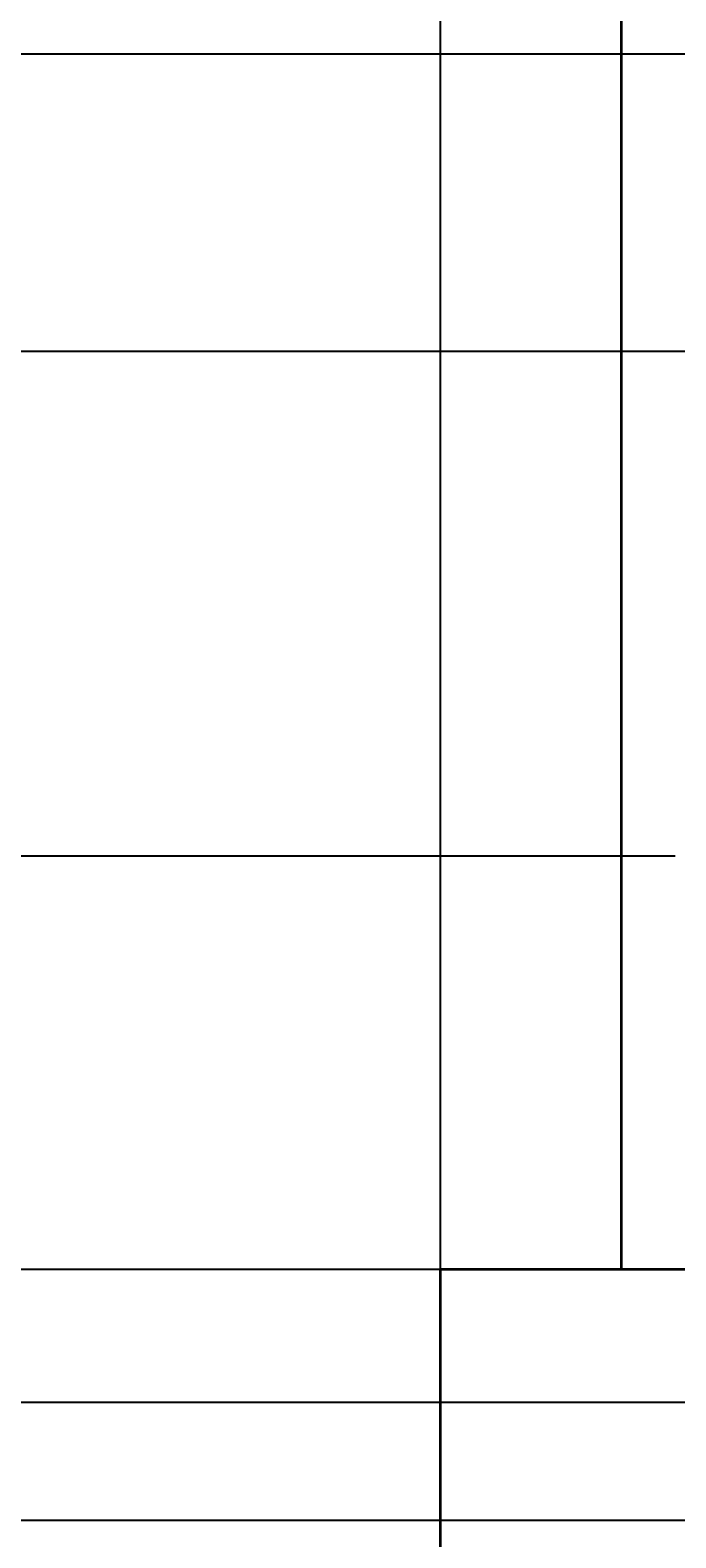
# Model space of a CAD drawing. Units: inches. Extents: x -145 to 510, y 5 to 386.
# Tile 10 of 25: x 18 to 75, y 177 to 308. Entities that reach past the tile are written whole.
import ezdxf

# ---------------------------------------------------------------- set-up
doc = ezdxf.new("R2010")
doc.units = ezdxf.units.IN
doc.header["$MEASUREMENT"] = 0
doc.layers.add('A-ANNO-DIMS', color=2, linetype='Continuous', lineweight=18)
doc.layers.add('A-ELEV', color=7, linetype='Continuous', lineweight=35)
doc.styles.get("Standard").update_dxf_attribs({"font": 'arial.ttf'})
doc.dimstyles.get("Standard").update_dxf_attribs({"dimtxt": 0.6875, "dimasz": 0.18, "dimexe": 0.18, "dimexo": 0.0625, "dimgap": 0.09, "dimtad": 0, "dimtih": 1, "dimtoh": 1, "dimdec": 4, "dimzin": 0, "dimdsep": 46, "dimlunit": 4, "dimtxsty": 'Standard', "dimcen": 0.09, "dimadec": 0, "dimazin": 0, "dimtfac": 1, "dimtdec": 4, "dimtofl": 0, "dimtmove": 0, "dimatfit": 3, "dimfxl": 1, "dimtolj": 1, "dimtzin": 0, "dimarcsym": 0})

# ---------------------------------------------------------------- blocks, each defined once
blk = doc.blocks.new('*D15')
at = {"layer": 'A-ANNO-DIMS', "color": 0, "lineweight": -2, "transparency": 16777216}
for p, q in [((69.78, 199.95), (69.78, 385.97)), ((69.96, 385.79), (80.93, 385.79)), ((94.96, 385.79), (83.98, 385.79)), ((95.14, 305.8), (95.14, 385.97))]:
    blk.add_line(p, q, dxfattribs=at)
at = {"layer": 'A-ANNO-DIMS', "color": 0, "transparency": 16777216}
for points in [[(69.96, 385.82), (69.96, 385.76), (69.78, 385.79)], [(94.96, 385.82), (94.96, 385.76), (95.14, 385.79)]]:
    blk.add_solid(points, dxfattribs=at)
at = {"layer": 'Defpoints', "color": 0, "transparency": 16777216}
for p in [(95.14, 385.79), (95.14, 305.74), (69.78, 199.89)]:
    blk.add_point(p, dxfattribs=at)
at = {"layer": 'A-ANNO-DIMS', "color": 0, "transparency": 16777216, "insert": (82.46, 385.79), "char_height": 0.688, "attachment_point": 5}
blk.add_mtext('\\A1;25.365', dxfattribs=at)
blk = doc.blocks.new('*D19')
at = {"layer": 'A-ANNO-DIMS', "color": 0, "lineweight": -2, "transparency": 16777216}
for p, q in [((478.76, 355.89), (-144.05, 355.89)), ((-143.87, 355.71), (-143.87, 218.33)), ((-143.87, 80.07), (-143.87, 217.45)), ((-114.04, 79.89), (-144.05, 79.89))]:
    blk.add_line(p, q, dxfattribs=at)
at = {"layer": 'A-ANNO-DIMS', "color": 0, "transparency": 16777216}
for points in [[(-143.9, 355.71), (-143.84, 355.71), (-143.87, 355.89)], [(-143.9, 80.07), (-143.84, 80.07), (-143.87, 79.89)]]:
    blk.add_solid(points, dxfattribs=at)
at = {"layer": 'Defpoints', "color": 0, "transparency": 16777216}
for p in [(-143.87, 355.89), (478.83, 355.89), (-113.97, 79.89)]:
    blk.add_point(p, dxfattribs=at)
at = {"layer": 'A-ANNO-DIMS', "color": 0, "transparency": 16777216, "insert": (-143.87, 217.89), "char_height": 0.688, "attachment_point": 5}
blk.add_mtext('\\A1;276', dxfattribs=at)
blk = doc.blocks.new('*D20')
at = {"layer": 'A-ANNO-DIMS', "color": 0, "lineweight": -2, "transparency": 16777216}
for p, q in [((53.94, 199.89), (-144.05, 199.89)), ((-143.87, 199.71), (-143.87, 140.33)), ((-143.87, 80.07), (-143.87, 139.45)), ((53.94, 79.89), (-144.05, 79.89))]:
    blk.add_line(p, q, dxfattribs=at)
at = {"layer": 'A-ANNO-DIMS', "color": 0, "transparency": 16777216}
for points in [[(-143.9, 199.71), (-143.84, 199.71), (-143.87, 199.89)], [(-143.9, 80.07), (-143.84, 80.07), (-143.87, 79.89)]]:
    blk.add_solid(points, dxfattribs=at)
at = {"layer": 'Defpoints', "color": 0, "transparency": 16777216}
for p in [(-143.87, 199.89), (54, 199.89), (54, 79.89)]:
    blk.add_point(p, dxfattribs=at)
at = {"layer": 'A-ANNO-DIMS', "color": 0, "transparency": 16777216, "insert": (-143.87, 139.89), "char_height": 0.688, "attachment_point": 5}
blk.add_mtext('\\A1;120', dxfattribs=at)
blk = doc.blocks.new('*D21')
at = {"layer": 'A-ANNO-DIMS', "color": 0, "lineweight": -2, "transparency": 16777216}
for p, q in [((34.21, 327.61), (-144.05, 327.61)), ((-143.87, 327.43), (-143.87, 264.19)), ((-143.87, 200.07), (-143.87, 263.31)), ((69.71, 199.89), (-144.05, 199.89))]:
    blk.add_line(p, q, dxfattribs=at)
at = {"layer": 'A-ANNO-DIMS', "color": 0, "transparency": 16777216}
for points in [[(-143.9, 327.43), (-143.84, 327.43), (-143.87, 327.61)], [(-143.9, 200.07), (-143.84, 200.07), (-143.87, 199.89)]]:
    blk.add_solid(points, dxfattribs=at)
at = {"layer": 'Defpoints', "color": 0, "transparency": 16777216}
for p in [(-143.87, 327.61), (34.27, 327.61), (69.78, 199.89)]:
    blk.add_point(p, dxfattribs=at)
at = {"layer": 'A-ANNO-DIMS', "color": 0, "transparency": 16777216, "insert": (-143.87, 263.75), "char_height": 0.688, "attachment_point": 5}
blk.add_mtext('\\A1;127.72', dxfattribs=at)
blk = doc.blocks.new('*D25')
at = {"layer": 'A-ANNO-DIMS', "color": 0, "lineweight": -2, "transparency": 16777216}
for p, q in [((74.44, 235.89), (-144.05, 235.89)), ((-143.87, 235.71), (-143.87, 218.33)), ((-143.87, 200.07), (-143.87, 217.45)), ((74.44, 199.89), (-144.05, 199.89))]:
    blk.add_line(p, q, dxfattribs=at)
at = {"layer": 'A-ANNO-DIMS', "color": 0, "transparency": 16777216}
for points in [[(-143.9, 235.71), (-143.84, 235.71), (-143.87, 235.89)], [(-143.9, 200.07), (-143.84, 200.07), (-143.87, 199.89)]]:
    blk.add_solid(points, dxfattribs=at)
at = {"layer": 'Defpoints', "color": 0, "transparency": 16777216}
for p in [(-143.87, 235.89), (74.51, 235.89), (74.51, 199.89)]:
    blk.add_point(p, dxfattribs=at)
at = {"layer": 'A-ANNO-DIMS', "color": 0, "transparency": 16777216, "insert": (-143.87, 217.89), "char_height": 0.688, "attachment_point": 5}
blk.add_mtext('\\A1;36', dxfattribs=at)
blk = doc.blocks.new('*D26')
at = {"layer": 'A-ANNO-DIMS', "color": 0, "lineweight": -2, "transparency": 16777216}
for p, q in [((95.08, 305.74), (-144.05, 305.74)), ((-143.87, 305.56), (-143.87, 253.26)), ((-143.87, 200.07), (-143.87, 252.38)), ((95.08, 199.89), (-144.05, 199.89))]:
    blk.add_line(p, q, dxfattribs=at)
at = {"layer": 'A-ANNO-DIMS', "color": 0, "transparency": 16777216}
for points in [[(-143.9, 305.56), (-143.84, 305.56), (-143.87, 305.74)], [(-143.9, 200.07), (-143.84, 200.07), (-143.87, 199.89)]]:
    blk.add_solid(points, dxfattribs=at)
at = {"layer": 'Defpoints', "color": 0, "transparency": 16777216}
for p in [(-143.87, 305.74), (95.14, 305.74), (95.14, 199.89)]:
    blk.add_point(p, dxfattribs=at)
at = {"layer": 'A-ANNO-DIMS', "color": 0, "transparency": 16777216, "insert": (-143.87, 252.82), "char_height": 0.688, "attachment_point": 5}
blk.add_mtext('\\A1;105.85', dxfattribs=at)
blk = doc.blocks.new('*D27')
at = {"layer": 'A-ANNO-DIMS', "color": 0, "lineweight": -2, "transparency": 16777216}
for p, q in [((244.23, 279.84), (-144.05, 279.84)), ((-143.87, 279.66), (-143.87, 240.31)), ((-143.87, 200.07), (-143.87, 239.43)), ((218.29, 199.89), (-144.05, 199.89))]:
    blk.add_line(p, q, dxfattribs=at)
at = {"layer": 'A-ANNO-DIMS', "color": 0, "transparency": 16777216}
for points in [[(-143.9, 279.66), (-143.84, 279.66), (-143.87, 279.84)], [(-143.9, 200.07), (-143.84, 200.07), (-143.87, 199.89)]]:
    blk.add_solid(points, dxfattribs=at)
at = {"layer": 'Defpoints', "color": 0, "transparency": 16777216}
for p in [(-143.87, 279.84), (244.29, 279.84), (218.36, 199.89)]:
    blk.add_point(p, dxfattribs=at)
at = {"layer": 'A-ANNO-DIMS', "color": 0, "transparency": 16777216, "insert": (-143.87, 239.87), "char_height": 0.688, "attachment_point": 5}
blk.add_mtext('\\A1;79.95', dxfattribs=at)
blk = doc.blocks.new('*D28')
at = {"layer": 'A-ANNO-DIMS', "color": 0, "lineweight": -2, "transparency": 16777216}
for p, q in [((244.23, 305.74), (-144.05, 305.74)), ((-143.87, 305.56), (-143.87, 293.23)), ((-143.87, 280.02), (-143.87, 292.35)), ((244.23, 279.84), (-144.05, 279.84))]:
    blk.add_line(p, q, dxfattribs=at)
at = {"layer": 'A-ANNO-DIMS', "color": 0, "transparency": 16777216}
for points in [[(-143.9, 305.56), (-143.84, 305.56), (-143.87, 305.74)], [(-143.9, 280.02), (-143.84, 280.02), (-143.87, 279.84)]]:
    blk.add_solid(points, dxfattribs=at)
at = {"layer": 'Defpoints', "color": 0, "transparency": 16777216}
for p in [(-143.87, 305.74), (244.29, 305.74), (244.29, 279.84)]:
    blk.add_point(p, dxfattribs=at)
at = {"layer": 'A-ANNO-DIMS', "color": 0, "transparency": 16777216, "insert": (-143.87, 292.79), "char_height": 0.688, "attachment_point": 5}
blk.add_mtext('\\A1;25.897', dxfattribs=at)
blk = doc.blocks.new('*D30')
at = {"layer": 'A-ANNO-DIMS', "color": 0, "lineweight": -2, "transparency": 16777216}
for p, q in [((210.73, 188.31), (-144.05, 188.31)), ((-143.87, 188.13), (-143.87, 183.61)), ((-143.87, 178.2), (-143.87, 182.72)), ((210.73, 178.02), (-144.05, 178.02))]:
    blk.add_line(p, q, dxfattribs=at)
at = {"layer": 'A-ANNO-DIMS', "color": 0, "transparency": 16777216}
for points in [[(-143.9, 188.13), (-143.84, 188.13), (-143.87, 188.31)], [(-143.9, 178.2), (-143.84, 178.2), (-143.87, 178.02)]]:
    blk.add_solid(points, dxfattribs=at)
at = {"layer": 'Defpoints', "color": 0, "transparency": 16777216}
for p in [(-143.87, 188.31), (210.8, 188.31), (210.8, 178.02)]:
    blk.add_point(p, dxfattribs=at)
at = {"layer": 'A-ANNO-DIMS', "color": 0, "transparency": 16777216, "insert": (-143.87, 183.16), "char_height": 0.688, "attachment_point": 5}
blk.add_mtext('\\A1;10.29', dxfattribs=at)
blk = doc.blocks.new('*D44')
at = {"layer": 'A-ANNO-DIMS', "color": 0, "lineweight": -2, "transparency": 16777216}
for p, q in [((34.27, 327.67), (34.27, 385.97)), ((34.45, 385.79), (42.92, 385.79)), ((53.82, 385.79), (45.35, 385.79)), ((54, 199.95), (54, 385.97))]:
    blk.add_line(p, q, dxfattribs=at)
at = {"layer": 'A-ANNO-DIMS', "color": 0, "transparency": 16777216}
for points in [[(34.45, 385.82), (34.45, 385.76), (34.27, 385.79)], [(53.82, 385.82), (53.82, 385.76), (54, 385.79)]]:
    blk.add_solid(points, dxfattribs=at)
at = {"layer": 'Defpoints', "color": 0, "transparency": 16777216}
for p in [(54, 385.79), (34.27, 327.61), (54, 199.89)]:
    blk.add_point(p, dxfattribs=at)
at = {"layer": 'A-ANNO-DIMS', "color": 0, "transparency": 16777216, "insert": (44.14, 385.79), "char_height": 0.688, "attachment_point": 5}
blk.add_mtext('\\A1;19.73', dxfattribs=at)

msp = doc.modelspace()

# ---------------------------------------------------------------- linework, layer by layer
at = {"layer": 'A-ELEV'}
for p, q in [((69.7763, 199.8905), (69.7763, 341.168)), ((54.0014, 79.8905), (54.0014, 199.8905)), ((218.3571, 199.8905), (54.0014, 199.8905))]:
    msp.add_line(p, q, dxfattribs=at)

# ---------------------------------------------------------------- dimensions: what is measured, and where the dimension line sits
at = {"layer": 'A-ANNO-DIMS'}
for base, p1, p2, override, picture, middle in [((54.0014, 385.7905), (34.2706, 327.6093), (54.0014, 199.8905), {"dimdec": 2, "dimlfac": 1, "dimrnd": 0, "dimzin": 0, "dimdsep": 46, "dimlunit": 2}, '*D44', (44.136, 385.7905)), ((95.1414, 385.7905), (69.7763, 199.8905), (95.1414, 305.7416), {"dimdec": 3, "dimlfac": 1, "dimrnd": 0, "dimzin": 0, "dimdsep": 46, "dimlunit": 2}, '*D15', (82.4589, 385.7905))]:
    dim = msp.add_linear_dim(base=base, p1=p1, p2=p2, dimstyle='Standard', override=override, dxfattribs=at)
    dim.commit()
    dim.dimension.update_dxf_attribs({"geometry": picture, "text_midpoint": middle})
for base, p1, p2, override, picture, middle in [((-143.8737, 355.8905), (-113.9737, 79.8905), (478.8263, 355.8905), {"dimdec": 0, "dimlfac": 1, "dimrnd": 0, "dimzin": 0, "dimdsep": 46, "dimlunit": 2}, '*D19', (-143.8737, 217.8905)), ((-143.8737, 327.6093), (69.7763, 199.8905), (34.2706, 327.6093), {"dimdec": 2, "dimlfac": 1, "dimrnd": 0, "dimzin": 0, "dimdsep": 46, "dimlunit": 2}, '*D21', (-143.8737, 263.7499)), ((-143.8737, 305.7416), (95.1414, 199.8905), (95.1414, 305.7416), {"dimdec": 2, "dimlfac": 1, "dimrnd": 0, "dimzin": 0, "dimdsep": 46, "dimlunit": 2}, '*D26', (-143.8737, 252.8161)), ((-143.8737, 305.7416), (244.2916, 279.8443), (244.2916, 305.7416), {"dimdec": 3, "dimlfac": 1, "dimrnd": 0, "dimzin": 0, "dimdsep": 46, "dimlunit": 2}, '*D28', (-143.8737, 292.793)), ((-143.8737, 279.8443), (218.3571, 199.8905), (244.2916, 279.8443), {"dimdec": 2, "dimlfac": 1, "dimrnd": 0, "dimzin": 0, "dimdsep": 46, "dimlunit": 2}, '*D27', (-143.8737, 239.8674)), ((-143.8737, 235.8905), (74.5073, 199.8905), (74.5073, 235.8905), {"dimdec": 0, "dimlfac": 1, "dimrnd": 0, "dimzin": 0, "dimdsep": 46, "dimlunit": 2}, '*D25', (-143.8737, 217.8905)), ((-143.8737, 199.8905), (54.0014, 79.8905), (54.0014, 199.8905), {"dimdec": 0, "dimlfac": 1, "dimrnd": 0, "dimzin": 0, "dimdsep": 46, "dimlunit": 2}, '*D20', (-143.8737, 139.8905)), ((-143.8737, 188.3087), (210.7973, 178.0195), (210.7973, 188.3087), {"dimdec": 2, "dimlfac": 1, "dimrnd": 0, "dimzin": 0, "dimdsep": 46, "dimlunit": 2}, '*D30', (-143.8737, 183.1641))]:
    dim = msp.add_linear_dim(base=base, p1=p1, p2=p2, angle=90, dimstyle='Standard', override=override, dxfattribs=at)
    dim.commit()
    dim.dimension.update_dxf_attribs({"geometry": picture, "text_midpoint": middle})

doc.saveas('drawing.dxf')
